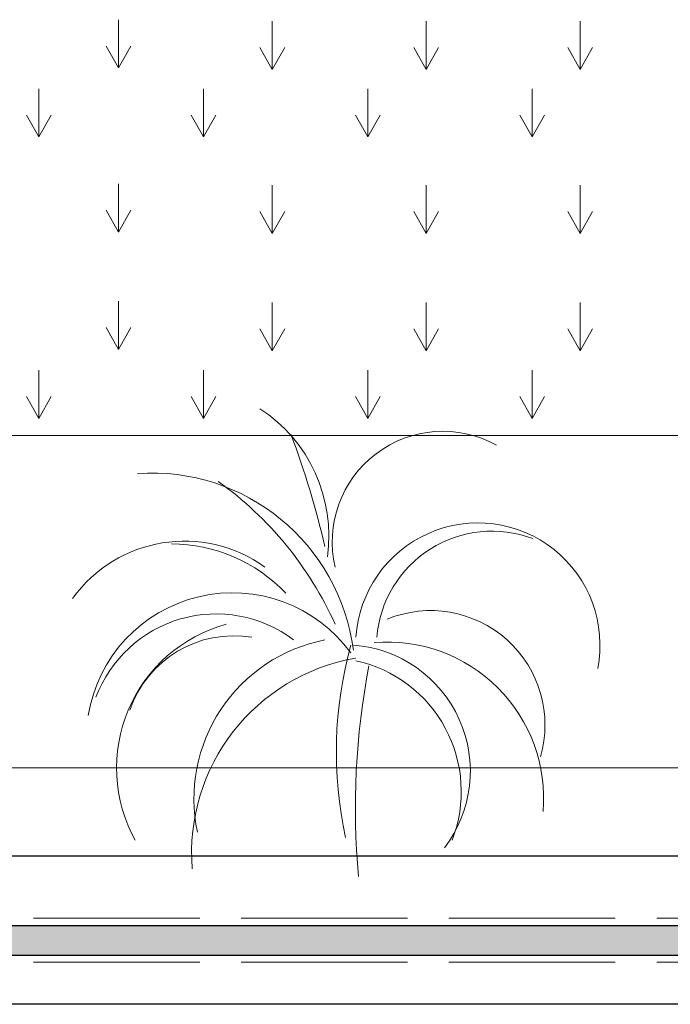
# Model space of a CAD drawing. Units: millimetres. Extents: x 595116 to 630915, y 909473 to 920225.
# Tile 93 of 134: x 629744 to 629791, y 919144 to 919215. Entities that reach past the tile are written whole.
import ezdxf

# ---------------------------------------------------------------- set-up
doc = ezdxf.new("R2010")
doc.units = ezdxf.units.MM
doc.linetypes.add('ACAD_ISO02W100', pattern=[15, 12, -3])
for name, color, linetype, lineweight in [('C-PROP', 7, 'Continuous', 25), ('C-PROP-REF', 240, 'ACAD_ISO02W100', 13), ('L-PLNT', 85, 'Continuous', 13)]:
    doc.layers.add(name, color=color, linetype=linetype, lineweight=lineweight)

# ---------------------------------------------------------------- blocks, each defined once
blk = doc.blocks.new('tree')
for centre, radius, start, end in [((629595.141, 919296.95), 5.184, 352.032, 57.0714), ((629569.835, 919289.496), 31.168, 13.149, 20.5076), ((629604.232, 919296.737), 3.791, 61.1347, 193.108), ((629594.259, 919292.132), 6.965, 7.4001, 94.0059), ((629589.446, 919288.922), 12.167, 24.2477, 54.3726), ((629605.429, 919293.205), 4.185, 348.9977, 176.315), ((629605.915, 919293.144), 3.963, 69.3845, 175.231), ((629595.377, 919292.044), 4.722, 54.2484, 144.2167), ((629594.88, 919291.171), 5.506, 43.8672, 89.4805), ((629597.025, 919289.989), 5.01, 36.0581, 170.6542), ((629596.464, 919289.874), 4.4, 52.9074, 159.3471), ((629603.809, 919290.469), 3.92, 343.886, 112.2662), ((629598.153, 919288.998), 5.103, 105.3576, 208.8973), ((629597.068, 919289.758), 3.768, 80.4816, 161.0664), ((629601.247, 919287.941), 5.545, 101.0419, 191.8692), ((629614.329, 919289.554), 13.748, 164.5925, 192.323), ((629600.849, 919288.894), 4.324, 322.5461, 85.805), ((629602.329, 919287.957), 5.355, 355.2141, 94.8217), ((629602.391, 919286.088), 6.769, 99.681, 184.5451), ((629626.813, 919287.645), 25.579, 169.0753, 185.2889), ((629600.275, 919288.191), 4.585, 338.7925, 77.6921)]:
    blk.add_arc(centre, radius, start, end)
blk = doc.blocks.new('LAWN-GRASS-TUFT')
blk.add_line((0.892, 3.485), (0.892, 0))
blk.add_lwpolyline([(0, 1.577), (0.892, 0), (1.785, 1.577)])

msp = doc.modelspace()

# ---------------------------------------------------------------- hatches: boundary and pattern name
at = {"layer": 'C-PROP'}
h = msp.add_hatch(color=256, dxfattribs=at)
h.dxf.hatch_style = 1
h.paths.add_polyline_path([(629809.541, 919149.555), (629625.041, 919149.555), (629625.041, 919147.413), (629809.541, 919147.413)])

# ---------------------------------------------------------------- linework, layer by layer
for p, q in [((629625.041, 919149.555), (629809.541, 919149.555)), ((629625.041, 919147.413), (629809.541, 919147.413))]:
    msp.add_line(p, q, dxfattribs=at)
msp.add_lwpolyline([(629809.541, 919143.864), (629625.041, 919143.864), (629625.041, 919154.587), (629809.541, 919154.587)], close=True, dxfattribs=at)
at = {"layer": 'C-PROP-REF'}
for p, q in [((629625.041, 919150.076), (629809.541, 919150.076)), ((629625.041, 919146.905), (629809.541, 919146.905))]:
    msp.add_line(p, q, dxfattribs=at)
at = {"layer": 'L-PLNT'}
for p, q in [((629535.274, 919184.917), (629800.951, 919184.917)), ((629511.274, 919160.917), (629824.951, 919160.917))]:
    msp.add_line(p, q, dxfattribs=at)

# ---------------------------------------------------------------- block references
for p in [(629750.277, 919211.424), (629761.391, 919211.325), (629772.505, 919211.325), (629783.619, 919211.325), (629744.542, 919206.447), (629756.415, 919206.447), (629768.288, 919206.447), (629780.161, 919206.447), (629750.277, 919199.586), (629761.391, 919199.487), (629772.505, 919199.487), (629783.619, 919199.487), (629750.277, 919191.116), (629761.391, 919191.017), (629772.505, 919191.017), (629783.619, 919191.017), (629744.542, 919186.14), (629756.415, 919186.14), (629768.288, 919186.14), (629780.161, 919186.14)]:
    msp.add_blockref('LAWN-GRASS-TUFT', p, dxfattribs=at)
at = {"layer": 'L-PLNT', "xscale": 2.107689410566463, "yscale": 2.107689410566463, "zscale": 2.107689410566463}
msp.add_blockref('tree', (-697235.57, -1018414.775), dxfattribs=at)

doc.saveas('drawing.dxf')
